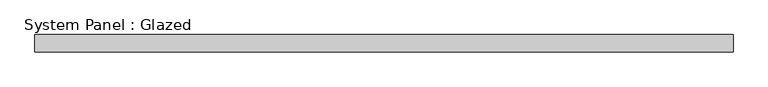
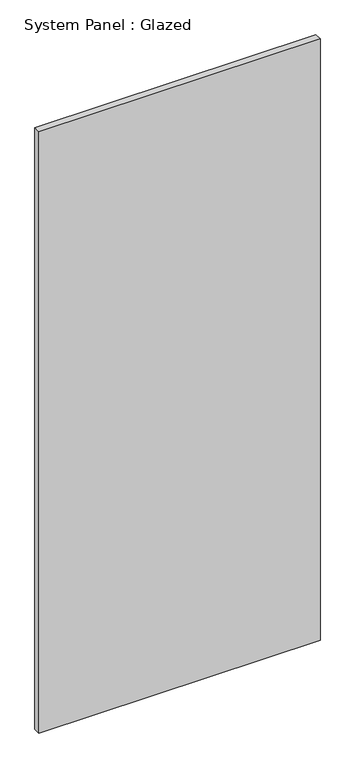
"""IFC4 building model written with IfcOpenShell, lengths in millimetres: plate geometry, System Panel : Glazed."""

from ifc_helpers import new_model, si_unit, origin, origin_with_axes, place, context, project, spatial, polyline, outline, extrude, source, transform, mapped, element, save


def system_panel_glazed_8311221f(model_context):
    return source(origin(), model_context, "Body", "SweptSolid", [
        extrude(outline(polyline([(511.175, 19.05), (-511.175, 19.05), (-511.175, 44.45), (511.175, 44.45), (511.175, 19.05)])), origin_with_axes(), (0.0, 0.0, 1.0), 2311.4),
    ])


if __name__ == "__main__":
    model = new_model("IFC4")
    model_context = context("Model", 3, world=origin())
    ifc_project = project(units=[si_unit("LENGTHUNIT", "METRE", prefix="MILLI")], contexts=[model_context])
    site = spatial("IfcSite", under=ifc_project)
    building = spatial("IfcBuilding", under=site)
    placement = place(None, origin())
    system_panel_glazed_shape = system_panel_glazed_8311221f(model_context)
    element("IfcPlate", 1, ObjectType="System Panel : Glazed", at=placement, inside=building, context=model_context, shape_type="MappedRepresentation", body=[
        mapped(system_panel_glazed_shape, transform((0.0, 0.0, 0.0), x_axis=(1.0, 0.0, 0.0), y_axis=(0.0, 1.0, 0.0), z_axis=(0.0, 0.0, 1.0))),
    ])
    save(model, "model.ifc")

# Revit data of these elements
# Type "System Panel : Glazed"
#   Construction Type Id = "GSP4R"
#   Analytic Construction = "1/8 in Pilkington single glazing"
#   Visual Light Transmittance = 0.9
#   Solar Heat Gain Coefficient = 0.86
#   Heat Transfer Coefficient (U) = 1.18115 BTU/(h·ft²·°F)
#   Define Thermal Properties by = 1
# Element 1 (IfcPlate, "System Panel : Glazed")
#   Materials on its faces: "Glass"
# Materials
#   "Glass": class "Glass", colour RGB 0 128 192, transparency 0.75, Description = "Soda Lime Glass", Cost = 0
